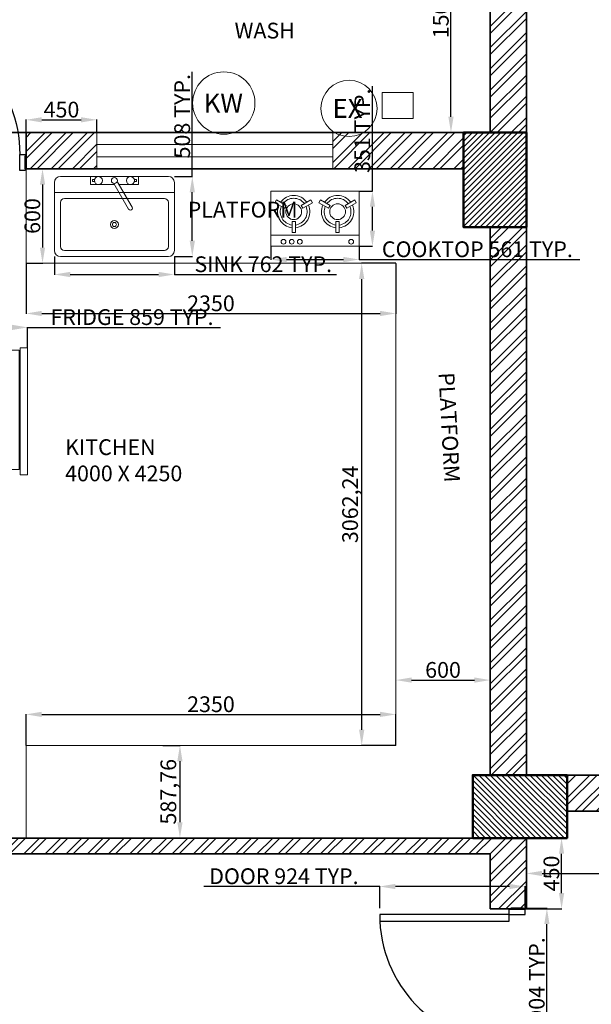
# Model space of a CAD drawing. Units: millimetres. Extents: x -3326 to 29338, y -16792 to 6002.
# Tile 10 of 21: x 8162 to 11795, y -3440 to 2813. Entities that reach past the tile are written whole.
import ezdxf

# ---------------------------------------------------------------- set-up
doc = ezdxf.new("R2010")
doc.units = ezdxf.units.MM
doc.header["$PDMODE"] = 35
doc.header["$PDSIZE"] = 5
for name, color, linetype, lineweight in [('A-ANNO-DIMS', 2, 'Continuous', 13), ('A-ANNO-SYMB', 7, 'Continuous', 18), ('A-AREA-IDEN', 7, 'Continuous', 18), ('A-COLS', 1, 'Continuous', 50), ('A-COLS-PATT', 251, 'Continuous', 13), ('A-DOOR', 3, 'Continuous', 25), ('A-EQPM', 9, 'Continuous', 18), ('A-FLOR-CASE', 30, 'Continuous', 18), ('A-FLOR-FIXT', 9, 'Continuous', 18), ('A-GLAZ', 4, 'Continuous', 18), ('A-WALL', 7, 'Continuous', 35), ('A-WALL-PATT', 252, 'Continuous', 13), ('txt', 7, 'Continuous', 18)]:
    doc.layers.add(name, color=color, linetype=linetype, lineweight=lineweight)
doc.styles.get("Standard").update_dxf_attribs({"font": 'arial.ttf'})
doc.dimstyles.new('ISO-25', dxfattribs={"dimtxt": 100, "dimasz": 100, "dimexe": 1.25, "dimexo": 0.625, "dimtad": 1, "dimtxsty": 'Standard', "dimcen": 2.5, "dimadec": 0, "dimazin": 0, "dimtfac": 1, "dimtmove": 0, "dimatfit": 3, "dimfxl": 1, "dimarcsym": 0})
pattern_1 = [(45, (-10476.65, 1e-12), (-67.35192, 67.35192), []), (45, (-10431.74, 1e-12), (-67.35192, 67.35192), [])]

# ---------------------------------------------------------------- blocks, each defined once
blk = doc.blocks.new('A$C0CE462CD')
for p, q in [((860, 100), (860, 0)), ((860, 0), (893.9, 0))]:
    blk.add_line(p, q)
for points in [[(860, 100), (860, 920), (818.4, 920), (818.4, 100)], [(0, 10), (6.1, 10), (6.1, 90), (0, 90)], [(893.9, 10), (900, 10), (900, 90), (893.9, 90)]]:
    blk.add_lwpolyline(points, close=True)
for points in [[(6.1, 0), (40, 0), (40, 100), (6.1, 100)], [(6.1, 100), (6.1, 0)], [(860, 100), (893.9, 100), (893.9, 0)]]:
    blk.add_lwpolyline(points)
blk.add_arc((859.1, 101.9), 819.1, 92.8508, 180.13091)
blk = doc.blocks.new('Sink-single - 30 in top')
blk.add_line((-15, -3.999996), (15, -3.999996))
for points in [[(-13.5, 0), (13.5, 0)], [(-15, -18.499996), (-15, -1.5)], [(15, -1.5), (15, -18.499996)], [(-13.5, -17.499996), (-13.5, -6.499996)], [(-12.5, -5.499996), (12.5, -5.499996)], [(13.5, -6.499996), (13.5, -17.499996)], [(12.5, -18.499996), (-12.5, -18.499996)], [(13.5, -19.999996), (-13.5, -19.999996)]]:
    blk.add_lwpolyline(points)
for radius in [1, 0.5]:
    blk.add_circle((0, -11.999996), radius)
for centre, radius, start, end in [((-13.5, -1.5), 1.5, 90, 180), ((13.5, -1.5), 1.5, 0, 90), ((-12.5, -6.499996), 1, 90, 180), ((12.5, -6.499996), 1, 0, 90), ((-13.5, -18.499996), 1.5, 180, 270), ((-12.5, -17.499996), 1, 180, 270), ((12.5, -17.499996), 1, 270, 0), ((13.5, -18.499996), 1.5, 270, 0)]:
    blk.add_arc(centre, radius, start, end)
blk = doc.blocks.new('Faucet - kit sink top')
for p, q in [((-5.5, -0.75), (-5.5, -1.25)), ((-4.94278, -0.75), (-5.5, -0.75)), ((-5.5, -1.25), (-4.94278, -1.25)), ((-0.14775, -1.7441), (3.56698, -8.1782)), ((4.43301, -7.6782), (0.71828, -1.2441)), ((4.94278, -0.75), (5.5, -0.75)), ((5.5, -1.25), (4.94278, -1.25)), ((5.5, -0.75), (5.5, -1.25))]:
    blk.add_line(p, q)
blk.add_lwpolyline([(-0.00587, -2), (-6, -2), (-6, 0), (6, 0), (6, -2), (1.15195, -2)])
for centre, radius in [((-4, -1), 1), ((4, -1), 1), ((0, -1), 0.75)]:
    blk.add_circle(centre, radius)
blk.add_arc((4, -7.9282), 0.5, 210, 30)
blk = doc.blocks.new('*D50')
at = {"layer": 'A-ANNO-DIMS', "color": 0, "lineweight": -2, "transparency": 16777216}
for p, q in [((11382.3, -2608.3), (11382.3, -2607.7)), ((11482.3, -2609), (17182.3, -2609)), ((17282.3, -2608.3), (17282.3, -2607.7))]:
    blk.add_line(p, q, dxfattribs=at)
at = {"layer": 'A-ANNO-DIMS', "color": 0, "transparency": 16777216}
for points in [[(11482.3, -2592.3), (11482.3, -2625.6), (11382.3, -2609)], [(17182.3, -2592.3), (17182.3, -2625.6), (17282.3, -2609)]]:
    blk.add_solid(points, dxfattribs=at)
at = {"layer": 'Defpoints', "color": 0, "transparency": 16777216}
for p in [(11382.3, -2609), (17282.3, -2609), (17282.3, -2609)]:
    blk.add_point(p, dxfattribs=at)
at = {"layer": 'A-ANNO-DIMS', "color": 0, "transparency": 16777216, "insert": (14332.3, -2557.3), "char_height": 100, "attachment_point": 5}
blk.add_mtext('5900', dxfattribs=at)
blk = doc.blocks.new('*D51')
at = {"layer": 'A-ANNO-DIMS', "color": 0, "lineweight": -2, "transparency": 16777216}
for p, q in [((11382.9, -2384), (11607, -2384)), ((11605.7, -2734), (11605.7, -2484)), ((11382.9, -2834), (11607, -2834))]:
    blk.add_line(p, q, dxfattribs=at)
at = {"layer": 'A-ANNO-DIMS', "color": 0, "transparency": 16777216}
for points in [[(11589.1, -2484), (11622.4, -2484), (11605.7, -2384)], [(11589.1, -2734), (11622.4, -2734), (11605.7, -2834)]]:
    blk.add_solid(points, dxfattribs=at)
at = {"layer": 'Defpoints', "color": 0, "transparency": 16777216}
for p in [(11382.3, -2384), (11605.7, -2384), (11382.3, -2834)]:
    blk.add_point(p, dxfattribs=at)
at = {"layer": 'A-ANNO-DIMS', "color": 0, "transparency": 16777216, "insert": (11554, -2609), "char_height": 100, "attachment_point": 5, "rotation": 90}
blk.add_mtext('450', dxfattribs=at)
blk = doc.blocks.new('*D121')
at = {"layer": 'A-ANNO-DIMS', "color": 0, "lineweight": -2, "transparency": 16777216}
for p, q in [((9071.8, -1796.2), (9181.4, -1796.2)), ((9180.2, -1896.2), (9180.2, -2284)), ((9071.8, -2384), (9181.4, -2384))]:
    blk.add_line(p, q, dxfattribs=at)
at = {"layer": 'A-ANNO-DIMS', "color": 0, "transparency": 16777216}
for points in [[(9163.5, -1896.2), (9196.8, -1896.2), (9180.2, -1796.2)], [(9163.5, -2284), (9196.8, -2284), (9180.2, -2384)]]:
    blk.add_solid(points, dxfattribs=at)
at = {"layer": 'Defpoints', "color": 0, "transparency": 16777216}
for p in [(9071.2, -1796.2), (9071.2, -2384), (9180.2, -2384)]:
    blk.add_point(p, dxfattribs=at)
at = {"layer": 'A-ANNO-DIMS', "color": 0, "transparency": 16777216, "insert": (9119.4, -2090.1), "char_height": 100, "attachment_point": 5, "rotation": 90}
blk.add_mtext('587,76', dxfattribs=at)
blk = doc.blocks.new('*D122')
at = {"layer": 'A-ANNO-DIMS', "color": 0, "lineweight": -2, "transparency": 16777216}
for p, q in [((10552.3, -1380.4), (10552.3, -1379.7)), ((10652.3, -1381), (11052.3, -1381)), ((11152.3, -1380.4), (11152.3, -1379.7))]:
    blk.add_line(p, q, dxfattribs=at)
at = {"layer": 'A-ANNO-DIMS', "color": 0, "transparency": 16777216}
for points in [[(10652.3, -1364.3), (10652.3, -1397.7), (10552.3, -1381)], [(11052.3, -1364.3), (11052.3, -1397.7), (11152.3, -1381)]]:
    blk.add_solid(points, dxfattribs=at)
at = {"layer": 'Defpoints', "color": 0, "transparency": 16777216}
for p in [(10552.3, -1381), (11152.3, -1381), (11152.3, -1381)]:
    blk.add_point(p, dxfattribs=at)
at = {"layer": 'A-ANNO-DIMS', "color": 0, "transparency": 16777216, "insert": (10852.3, -1329.3), "char_height": 100, "attachment_point": 5}
blk.add_mtext('600', dxfattribs=at)
blk = doc.blocks.new('*D123')
at = {"layer": 'A-ANNO-DIMS', "color": 0, "lineweight": -2, "transparency": 16777216}
for p, q in [((8202.9, 1866), (8308, 1866)), ((8306.8, 1766), (8306.8, 1366)), ((8202.9, 1266), (8308, 1266))]:
    blk.add_line(p, q, dxfattribs=at)
at = {"layer": 'A-ANNO-DIMS', "color": 0, "transparency": 16777216}
for points in [[(8290.1, 1766), (8323.5, 1766), (8306.8, 1866)], [(8290.1, 1366), (8323.5, 1366), (8306.8, 1266)]]:
    blk.add_solid(points, dxfattribs=at)
at = {"layer": 'Defpoints', "color": 0, "transparency": 16777216}
for p in [(8202.3, 1866), (8202.3, 1266), (8306.8, 1266)]:
    blk.add_point(p, dxfattribs=at)
at = {"layer": 'A-ANNO-DIMS', "color": 0, "transparency": 16777216, "insert": (8255.1, 1566), "char_height": 100, "attachment_point": 5, "rotation": 90}
blk.add_mtext('600', dxfattribs=at)
blk = doc.blocks.new('*D124')
at = {"layer": 'A-ANNO-DIMS', "color": 0, "lineweight": -2, "transparency": 16777216}
for p, q in [((8202.3, 1265.4), (8202.3, 945.9)), ((10552.3, 1265.4), (10552.3, 945.9)), ((8302.3, 947.1), (10452.3, 947.1))]:
    blk.add_line(p, q, dxfattribs=at)
at = {"layer": 'A-ANNO-DIMS', "color": 0, "transparency": 16777216}
for points in [[(8302.3, 963.8), (8302.3, 930.5), (8202.3, 947.1)], [(10452.3, 963.8), (10452.3, 930.5), (10552.3, 947.1)]]:
    blk.add_solid(points, dxfattribs=at)
at = {"layer": 'Defpoints', "color": 0, "transparency": 16777216}
for p in [(8202.3, 1266), (10552.3, 1266), (10552.3, 947.1)]:
    blk.add_point(p, dxfattribs=at)
at = {"layer": 'A-ANNO-DIMS', "color": 0, "transparency": 16777216, "insert": (9377.3, 998.8), "char_height": 100, "attachment_point": 5}
blk.add_mtext('2350', dxfattribs=at)
blk = doc.blocks.new('*D125')
at = {"layer": 'A-ANNO-DIMS', "color": 0, "lineweight": -2, "transparency": 16777216}
for p, q in [((8202.3, -1795.6), (8202.3, -1597.6)), ((8302.3, -1598.9), (10452.3, -1598.9)), ((10552.3, -1795.6), (10552.3, -1597.6))]:
    blk.add_line(p, q, dxfattribs=at)
at = {"layer": 'A-ANNO-DIMS', "color": 0, "transparency": 16777216}
for points in [[(8302.3, -1582.2), (8302.3, -1615.5), (8202.3, -1598.9)], [(10452.3, -1582.2), (10452.3, -1615.5), (10552.3, -1598.9)]]:
    blk.add_solid(points, dxfattribs=at)
at = {"layer": 'Defpoints', "color": 0, "transparency": 16777216}
for p in [(10552.3, -1598.9), (8202.3, -1796.2), (10552.3, -1796.2)]:
    blk.add_point(p, dxfattribs=at)
at = {"layer": 'A-ANNO-DIMS', "color": 0, "transparency": 16777216, "insert": (9377.3, -1547.1), "char_height": 100, "attachment_point": 5}
blk.add_mtext('2350', dxfattribs=at)
blk = doc.blocks.new('*D126')
at = {"layer": 'A-ANNO-DIMS', "color": 0, "lineweight": -2, "transparency": 16777216}
for p, q in [((10551.7, 1266), (10334, 1266)), ((10335.3, -1696.2), (10335.3, 1166)), ((10551.7, -1796.2), (10334, -1796.2))]:
    blk.add_line(p, q, dxfattribs=at)
at = {"layer": 'A-ANNO-DIMS', "color": 0, "transparency": 16777216}
for points in [[(10318.6, 1166), (10352, 1166), (10335.3, 1266)], [(10318.6, -1696.2), (10352, -1696.2), (10335.3, -1796.2)]]:
    blk.add_solid(points, dxfattribs=at)
at = {"layer": 'Defpoints', "color": 0, "transparency": 16777216}
for p in [(10335.3, 1266), (10552.3, 1266), (10552.3, -1796.2)]:
    blk.add_point(p, dxfattribs=at)
at = {"layer": 'A-ANNO-DIMS', "color": 0, "transparency": 16777216, "insert": (10274.6, -265.1), "char_height": 100, "attachment_point": 5, "rotation": 90}
blk.add_mtext('3062,24', dxfattribs=at)
blk = doc.blocks.new('*D127')
at = {"layer": 'A-ANNO-DIMS', "color": 0, "lineweight": -2, "transparency": 16777216}
for p, q in [((11151.7, 3596), (10901.5, 3596)), ((10902.7, 2196), (10902.7, 3496)), ((11151.7, 2096), (10901.5, 2096))]:
    blk.add_line(p, q, dxfattribs=at)
at = {"layer": 'A-ANNO-DIMS', "color": 0, "transparency": 16777216}
for points in [[(10886.1, 3496), (10919.4, 3496), (10902.7, 3596)], [(10886.1, 2196), (10919.4, 2196), (10902.7, 2096)]]:
    blk.add_solid(points, dxfattribs=at)
at = {"layer": 'Defpoints', "color": 0, "transparency": 16777216}
for p in [(10902.7, 3596), (11152.3, 3596), (11152.3, 2096)]:
    blk.add_point(p, dxfattribs=at)
at = {"layer": 'A-ANNO-DIMS', "color": 0, "transparency": 16777216, "insert": (10851.1, 2846), "char_height": 100, "attachment_point": 5, "rotation": 90}
blk.add_mtext('1500', dxfattribs=at)
blk = doc.blocks.new('*D144')
at = {"layer": 'A-ANNO-DIMS', "color": 0, "lineweight": -2, "transparency": 16777216}
for p, q in [((8202.3, 2096.7), (8202.3, 2178.4)), ((8302.3, 2177.1), (8552.3, 2177.1)), ((8652.3, 2096.7), (8652.3, 2178.4))]:
    blk.add_line(p, q, dxfattribs=at)
at = {"layer": 'A-ANNO-DIMS', "color": 0, "transparency": 16777216}
for points in [[(8302.3, 2193.8), (8302.3, 2160.5), (8202.3, 2177.1)], [(8552.3, 2193.8), (8552.3, 2160.5), (8652.3, 2177.1)]]:
    blk.add_solid(points, dxfattribs=at)
at = {"layer": 'Defpoints', "color": 0, "transparency": 16777216}
for p in [(8652.3, 2177.1), (8202.3, 2096), (8652.3, 2096)]:
    blk.add_point(p, dxfattribs=at)
at = {"layer": 'A-ANNO-DIMS', "color": 0, "transparency": 16777216, "insert": (8427.3, 2228.8), "char_height": 100, "attachment_point": 5}
blk.add_mtext('450', dxfattribs=at)
blk = doc.blocks.new('COOKTOP-TWO-BURNER')
for p, q in [((561.3, 350.8), (0, 350.8)), ((0, 0), (0, 350.8)), ((561.3, 0), (561.3, 350.8)), ((26.1, 276.2), (36.6, 294.4)), ((86.6, 241.2), (26.1, 276.2)), ((97.2, 259.4), (36.6, 294.4)), ((86.6, 241.2), (97.2, 259.4)), ((193, 259.4), (253.6, 294.3)), ((193, 259.4), (203.5, 241.1)), ((203.5, 241.1), (264.1, 276.1)), ((253.6, 294.3), (264.1, 276.1)), ((305, 276.2), (315.6, 294.4)), ((365.6, 241.2), (305, 276.2)), ((376.1, 259.4), (315.6, 294.4)), ((365.6, 241.2), (376.1, 259.4)), ((472, 259.4), (532.5, 294.3)), ((472, 259.4), (482.5, 241.1)), ((482.5, 241.1), (543, 276.1)), ((532.5, 294.3), (543, 276.1)), ((134.5, 158.1), (134.5, 88.2)), ((155.6, 158.1), (134.5, 158.1)), ((155.6, 158.1), (155.5, 88.2)), ((413.5, 158.1), (413.4, 88.2)), ((434.5, 158.1), (413.5, 158.1)), ((434.5, 158.1), (434.5, 88.2)), ((561.3, 70.2), (0, 70.2)), ((155.5, 88.2), (134.5, 88.2)), ((434.5, 88.2), (413.4, 88.2)), ((561.3, 0), (0, 0))]:
    blk.add_line(p, q)
at = {"extrusion": (0, 0, -1)}
for centre, major_axis, start_param, end_param in [((145.1, 219.6), (-0.2, 102.8), -0.942584, 0.946692), ((424, 219.6), (0, 102.8), -0.944011, 0.945266), ((145.1, 219.6), (-0.1, 102.8), 3.2451, 5.134376), ((145.1, 219.6), (-60.3, 60.3), 4.051123, 5.898002), ((145.1, 219.6), (-60.3, 60.3), 6.145519, 7.992397), ((145.1, 219.6), (-35.5, 35.5), 2.356194490192311, 8.639379797371898), ((145.1, 219.6), (0.1, 102.8), 1.148752, 3.038029), ((145.1, 219.6), (60.3, 60.3), 0.385932, 2.23281), ((424, 219.6), (0, 102.8), 3.244173, 5.13345), ((424, 219.6), (60.3, 60.3), 2.480327, 4.327205), ((424, 219.6), (-60.3, 60.3), 6.145519, 7.992397), ((424, 219.6), (-35.5, 35.5), 2.356194490192306, 8.639379797371893), ((424, 219.6), (0.1, 102.8), 1.14879, 3.038067), ((424, 219.6), (60.3, 60.3), 0.385932, 2.23281), ((79.9, 28.7), (-10.8, 10.8), 2.356194490192189, 8.639379797371776), ((132.6, 28.7), (-10.8, 10.8), 2.356194490192189, 8.639379797371776), ((184.2, 28.7), (-10.8, 10.8), 2.356194490192189, 8.639379797371776), ((510, 28.7), (-10.8, 10.8), 2.356194490192189, 8.639379797371776)]:
    blk.add_ellipse(centre, major_axis=major_axis, ratio=1, start_param=start_param, end_param=end_param, dxfattribs=at)
blk = doc.blocks.new('REFRIGERATOR-PLAN')
for points in [[(0, 791.3), (804.9, 791.3), (804.9, 34.9), (0, 34.9)], [(812.5, 807.8), (859.3, 807.8), (859.3, 0), (812.5, 0)]]:
    blk.add_lwpolyline(points, close=True)
blk = doc.blocks.new('TAG-KW')
blk.add_circle((198.2, 198.2), 198.2)
at = {"insert": (70.3, 258.2), "char_height": 120, "attachment_point": 1}
blk.add_mtext_dynamic_manual_height_columns('KW', width=376.575, gutter_width=12.5, heights=[0], dxfattribs=at)
blk = doc.blocks.new('GLAZ-1500x80')
for p, q in [((0, 80), (1500, 80)), ((0, 0), (1500, 0))]:
    blk.add_line(p, q)
blk = doc.blocks.new('*D195')
at = {"layer": 'A-ANNO-DIMS', "color": 0, "lineweight": -2, "transparency": 16777216}
for p, q in [((10450.2, -2691.8), (9331.5, -2691.8)), ((10450.2, -2829.8), (10450.2, -2690.6)), ((11273.9, -2691.8), (10550.2, -2691.8)), ((11373.9, -2829.8), (11373.9, -2690.6))]:
    blk.add_line(p, q, dxfattribs=at)
at = {"layer": 'A-ANNO-DIMS', "color": 0, "transparency": 16777216}
for points in [[(10550.2, -2675.2), (10550.2, -2708.5), (10450.2, -2691.8)], [(11273.9, -2675.2), (11273.9, -2708.5), (11373.9, -2691.8)]]:
    blk.add_solid(points, dxfattribs=at)
at = {"layer": 'Defpoints', "color": 0, "transparency": 16777216}
for p in [(10450.2, -2691.8), (10450.2, -2830.4), (11373.9, -2830.4)]:
    blk.add_point(p, dxfattribs=at)
at = {"layer": 'A-ANNO-DIMS', "color": 0, "transparency": 16777216, "insert": (9840.8, -2639.5), "char_height": 100, "attachment_point": 5}
blk.add_mtext('DOOR 924 TYP.', dxfattribs=at)
blk = doc.blocks.new('*D196')
at = {"layer": 'A-ANNO-DIMS', "color": 0, "lineweight": -2, "transparency": 16777216}
for p, q in [((11374.5, -2830.4), (11513.7, -2830.4)), ((11512.5, -3634.1), (11512.5, -2930.4)), ((11374.5, -3734.1), (11513.7, -3734.1))]:
    blk.add_line(p, q, dxfattribs=at)
at = {"layer": 'A-ANNO-DIMS', "color": 0, "transparency": 16777216}
for points in [[(11495.8, -2930.4), (11529.1, -2930.4), (11512.5, -2830.4)], [(11495.8, -3634.1), (11529.1, -3634.1), (11512.5, -3734.1)]]:
    blk.add_solid(points, dxfattribs=at)
at = {"layer": 'Defpoints', "color": 0, "transparency": 16777216}
for p in [(11373.9, -2830.4), (11512.5, -2830.4), (11373.9, -3734.1)]:
    blk.add_point(p, dxfattribs=at)
at = {"layer": 'A-ANNO-DIMS', "color": 0, "transparency": 16777216, "insert": (11460.8, -3282.2), "char_height": 100, "attachment_point": 5, "rotation": 90}
blk.add_mtext('904 TYP.', dxfattribs=at)
blk = doc.blocks.new('*D221')
at = {"layer": 'A-ANNO-DIMS', "color": 0, "lineweight": -2, "transparency": 16777216}
for p, q in [((8382.6, 1308.4), (8382.6, 1193.4)), ((9144.6, 1308.4), (9144.6, 1193.4)), ((8482.6, 1194.7), (9044.6, 1194.7)), ((9144.6, 1194.7), (10174.7, 1194.7))]:
    blk.add_line(p, q, dxfattribs=at)
at = {"layer": 'A-ANNO-DIMS', "color": 0, "transparency": 16777216}
for points in [[(8482.6, 1211.3), (8482.6, 1178), (8382.6, 1194.7)], [(9044.6, 1211.3), (9044.6, 1178), (9144.6, 1194.7)]]:
    blk.add_solid(points, dxfattribs=at)
at = {"layer": 'Defpoints', "color": 0, "transparency": 16777216}
for p in [(8382.6, 1309), (9144.6, 1309), (9144.6, 1194.7)]:
    blk.add_point(p, dxfattribs=at)
at = {"layer": 'A-ANNO-DIMS', "color": 0, "transparency": 16777216, "insert": (9709.7, 1247), "char_height": 100, "attachment_point": 5}
blk.add_mtext('SINK 762 TYP.', dxfattribs=at)
blk = doc.blocks.new('*D222')
at = {"layer": 'A-ANNO-DIMS', "color": 0, "lineweight": -2, "transparency": 16777216}
for p, q in [((9258.9, 1817), (9258.9, 2482.7)), ((9145.2, 1817), (9260.2, 1817)), ((9258.9, 1409), (9258.9, 1717)), ((9145.2, 1309), (9260.2, 1309))]:
    blk.add_line(p, q, dxfattribs=at)
at = {"layer": 'A-ANNO-DIMS', "color": 0, "transparency": 16777216}
for points in [[(9242.2, 1717), (9275.6, 1717), (9258.9, 1817)], [(9242.2, 1409), (9275.6, 1409), (9258.9, 1309)]]:
    blk.add_solid(points, dxfattribs=at)
at = {"layer": 'Defpoints', "color": 0, "transparency": 16777216}
for p in [(9144.6, 1817), (9258.9, 1817), (9144.6, 1309)]:
    blk.add_point(p, dxfattribs=at)
at = {"layer": 'A-ANNO-DIMS', "color": 0, "transparency": 16777216, "insert": (9207.2, 2199.8), "char_height": 100, "attachment_point": 5, "rotation": 90}
blk.add_mtext('508 TYP.', dxfattribs=at)
blk = doc.blocks.new('*D231')
at = {"layer": 'A-ANNO-DIMS', "color": 0, "lineweight": -2, "transparency": 16777216}
for p, q in [((9758.2, 1373.4), (9758.2, 1288.5)), ((10319.5, 1373.4), (10319.5, 1288.5)), ((9858.2, 1289.8), (10219.5, 1289.8)), ((10319.5, 1289.8), (11721.4, 1289.8))]:
    blk.add_line(p, q, dxfattribs=at)
at = {"layer": 'A-ANNO-DIMS', "color": 0, "transparency": 16777216}
for points in [[(9858.2, 1306.4), (9858.2, 1273.1), (9758.2, 1289.8)], [(10219.5, 1306.4), (10219.5, 1273.1), (10319.5, 1289.8)]]:
    blk.add_solid(points, dxfattribs=at)
at = {"layer": 'Defpoints', "color": 0, "transparency": 16777216}
for p in [(9758.2, 1374), (10319.5, 1374), (10319.5, 1289.8)]:
    blk.add_point(p, dxfattribs=at)
at = {"layer": 'A-ANNO-DIMS', "color": 0, "transparency": 16777216, "insert": (11070.5, 1342.1), "char_height": 100, "attachment_point": 5}
blk.add_mtext('COOKTOP 561 TYP.', dxfattribs=at)
blk = doc.blocks.new('*D232')
at = {"layer": 'A-ANNO-DIMS', "color": 0, "lineweight": -2, "transparency": 16777216}
for p, q in [((10403.7, 1724.8), (10403.7, 2390.4)), ((10320.1, 1724.8), (10405, 1724.8)), ((10403.7, 1474), (10403.7, 1624.8)), ((10320.1, 1374), (10405, 1374))]:
    blk.add_line(p, q, dxfattribs=at)
at = {"layer": 'A-ANNO-DIMS', "color": 0, "transparency": 16777216}
for points in [[(10387, 1624.8), (10420.4, 1624.8), (10403.7, 1724.8)], [(10387, 1474), (10420.4, 1474), (10403.7, 1374)]]:
    blk.add_solid(points, dxfattribs=at)
at = {"layer": 'Defpoints', "color": 0, "transparency": 16777216}
for p in [(10319.5, 1724.8), (10403.7, 1724.8), (10319.5, 1374)]:
    blk.add_point(p, dxfattribs=at)
at = {"layer": 'A-ANNO-DIMS', "color": 0, "transparency": 16777216, "insert": (10352, 2107.6), "char_height": 100, "attachment_point": 5, "rotation": 90}
blk.add_mtext('351 TYP.', dxfattribs=at)
blk = doc.blocks.new('*D233')
at = {"layer": 'A-ANNO-DIMS', "color": 0, "lineweight": -2, "transparency": 16777216}
for p, q in [((7352.6, 730.5), (7352.6, 860.1)), ((7452.6, 858.8), (8111.9, 858.8)), ((8211.9, 730.5), (8211.9, 860.1)), ((8211.9, 858.8), (9438.5, 858.8))]:
    blk.add_line(p, q, dxfattribs=at)
at = {"layer": 'A-ANNO-DIMS', "color": 0, "transparency": 16777216}
for points in [[(7452.6, 875.5), (7452.6, 842.1), (7352.6, 858.8)], [(8111.9, 875.5), (8111.9, 842.1), (8211.9, 858.8)]]:
    blk.add_solid(points, dxfattribs=at)
at = {"layer": 'Defpoints', "color": 0, "transparency": 16777216}
for p in [(8211.9, 858.8), (7352.6, 729.9), (8211.9, 729.9)]:
    blk.add_point(p, dxfattribs=at)
at = {"layer": 'A-ANNO-DIMS', "color": 0, "transparency": 16777216, "insert": (8875.2, 911.1), "char_height": 100, "attachment_point": 5}
blk.add_mtext('FRIDGE 859 TYP.', dxfattribs=at)

msp = doc.modelspace()

# ---------------------------------------------------------------- hatches: boundary and pattern name
at = {"layer": 'A-COLS-PATT'}
h = msp.add_hatch(dxfattribs=at)
h.set_pattern_fill('ANSI31', color=256, scale=8)
h.set_pattern_definition([(45, (-30739, 8703.052), (-17.960512, 17.960512), [])])
h.paths.add_polyline_path([(10982.301, 1496.048), (11382.301, 1496.048), (11382.301, 2096.048), (10982.301, 2096.048)])
h = msp.add_hatch(dxfattribs=at)
h.set_pattern_fill('ANSI31', color=256, scale=8, angle=-90)
h.set_pattern_definition([(315, (18247.866, 39737.347), (17.960512, 17.960512), [])])
h.paths.add_polyline_path([(11040.861, -1983.952), (11040.861, -2383.952), (11640.861, -2383.952), (11640.861, -1983.952)])
at = {"layer": 'A-WALL-PATT'}
h = msp.add_hatch(dxfattribs=at)
h.set_pattern_fill('ANSI32', color=256, scale=10)
h.set_pattern_definition(pattern_1)
h.paths.add_polyline_path([(12212.301, -1983.952), (11640.861, -1983.952), (11640.861, -2213.952), (12212.301, -2213.952)])
h.paths.add_polyline_path([(14712.301, -1983.952), (14012.301, -1983.952), (14012.301, -2213.952), (14712.301, -2213.952)])
h.paths.add_polyline_path([(17012.301, -1983.952), (16512.301, -1983.952), (16512.301, -2213.952), (17012.301, -2213.952)])
h.paths.add_polyline_path([(11382.301, -2383.952), (11040.861, -2383.952), (7302.301, -2383.952), (7302.301, -1935.766), (7217.026, -1935.766), (7202.301, -1933.952), (7202.301, -2483.952), (7302.301, -2483.952), (11152.301, -2483.952), (11152.301, -2833.952), (11283.549, -2833.952), (11283.549, -2830.395), (11363.875, -2830.395), (11382.301, -2833.952)])
h.paths.add_polyline_path([(11382.301, -3733.952), (11363.875, -3733.952), (11363.875, -3734.058), (11283.549, -3734.058), (11152.301, -3733.952), (11152.301, -6450.401), (11382.301, -6450.401)])
h.paths.add_polyline_path([(13462.301, -6450.401), (12606.738, -6450.401), (11382.301, -6450.401), (11382.301, -6680.401), (12606.738, -6680.401), (13462.301, -6680.401)])
h.paths.add_polyline_path([(11382.301, -7050.401), (11152.301, -7050.401), (11152.301, -8810.401), (11382.301, -8810.401)])
h.paths.add_polyline_path([(13462.301, -8980.401), (11751.174, -8980.401), (11751.174, -9210.401), (13462.301, -9210.401)])
h.paths.add_polyline_path([(13962.301, -6850.401), (13732.301, -6850.401), (13732.301, -7350.401), (13962.301, -7350.401)])
h.paths.add_polyline_path([(13962.301, -8309.482), (13732.301, -8309.482), (13732.301, -8809.482), (13962.301, -8809.482)])
h.paths.add_polyline_path([(15712.301, -12533.952), (12902.301, -12533.952), (12902.301, -12763.952), (15712.301, -12763.952)])
h.paths.add_polyline_path([(11508.301, -9211.585), (11382.301, -9211.585), (11152.301, -9211.585), (11152.301, -11033.952), (10952.301, -11033.952), (10952.301, -11263.952), (11152.301, -11263.952), (11152.301, -12361.585), (11508.301, -12361.585)])
h.paths.add_polyline_path([(12002.301, -12533.952), (11902.301, -12533.952), (11902.301, -12761.585), (11152.301, -12761.585), (11152.301, -12763.952), (11902.301, -12763.952), (12002.301, -12763.952)])
h.paths.add_polyline_path([(17112.301, -12533.952), (16912.301, -12533.952), (16912.301, -12763.952), (17112.301, -12763.952)])
h.paths.add_polyline_path([(11382.301, 3596.048), (11152.301, 3596.048), (11152.301, 2096.048), (11382.301, 2096.048)])
h.paths.add_polyline_path([(11382.301, 1496.048), (11152.301, 1496.048), (11152.301, -1983.952), (11382.301, -1983.952)])
h = msp.add_hatch(dxfattribs=at)
h.set_pattern_fill('ANSI32', color=256, scale=10)
h.set_pattern_definition(pattern_1)
h.paths.add_polyline_path([(8652.301, 2096.048), (8202.301, 2096.048), (8202.301, 1866.048), (8652.301, 1866.048)])
h.paths.add_polyline_path([(10982.301, 2096.048), (10152.301, 2096.048), (10152.301, 1866.048), (10982.301, 1866.048)])

# ---------------------------------------------------------------- linework, layer by layer
at = {"layer": 'A-ANNO-SYMB'}
msp.add_circle((10254.723, 2249.364), 178.636, dxfattribs=at)
at = {"layer": 'A-COLS'}
for points in [[(10982.301, 2096.048), (11382.301, 2096.048), (11382.301, 1496.048), (10982.301, 1496.048)], [(11640.861, -1983.952), (11640.861, -2383.952), (11040.861, -2383.952), (11040.861, -1983.952)]]:
    msp.add_lwpolyline(points, close=True, dxfattribs=at)
at = {"layer": 'A-EQPM'}
msp.add_lwpolyline([(10465.362, 2349.703), (10661.811, 2349.703), (10661.811, 2184.867), (10465.362, 2184.867)], close=True, dxfattribs=at)
at = {"layer": 'A-FLOR-CASE'}
for p, q in [((8202.301, 1866.048), (8202.301, 1266.048)), ((8202.301, 1266.048), (10552.301, 1266.048)), ((10552.301, 1266.048), (10552.301, -1796.189)), ((10552.301, -1796.189), (8202.301, -1796.189)), ((8202.301, -1796.189), (8202.301, -2383.952))]:
    msp.add_line(p, q, dxfattribs=at)
at = {"layer": 'A-GLAZ'}
for p, q in [((8652.301, 2096.048), (8652.301, 1866.048)), ((10152.301, 2096.048), (10152.301, 1866.048))]:
    msp.add_line(p, q, dxfattribs=at)
at = {"layer": 'A-WALL'}
for p, q in [((11152.301, 3596.048), (11152.301, 2096.048)), ((11382.301, 3596.048), (11382.301, -1983.952)), ((10982.301, 2096.048), (7302.301, 2096.048)), ((8202.301, 2096.048), (8202.301, 1866.048)), ((10982.301, 1866.048), (8202.301, 1866.048)), ((11152.301, 1496.048), (11152.301, -1983.952)), ((17012.301, -1983.952), (11640.861, -1983.952)), ((17012.301, -2213.952), (11640.861, -2213.952)), ((11152.301, -2383.952), (7302.301, -2383.952)), ((11382.301, -2383.952), (11382.301, -2833.952)), ((11152.301, -2483.952), (7302.301, -2483.952)), ((11152.301, -2483.952), (11152.301, -2833.952)), ((11382.301, -2833.952), (11152.301, -2833.952))]:
    msp.add_line(p, q, dxfattribs=at)

# ---------------------------------------------------------------- block references
at = {"layer": 'A-ANNO-SYMB'}
msp.add_blockref('TAG-KW', (9260.815, 2085.197), dxfattribs=at)
at = {"layer": 'A-DOOR', "xscale": -1}
msp.add_blockref('A$C0CE462CD', (8202.301, 1856.048), dxfattribs=at)
at = {"layer": 'A-DOOR', "xscale": 1.004070386304363, "yscale": 1.004070386304363, "zscale": 1.004070386304363, "rotation": 90.00000000000003}
msp.add_blockref('A$C0CE462CD', (11373.915, -3734.058), dxfattribs=at)
at = {"layer": 'A-EQPM'}
for name, p in [('COOKTOP-TWO-BURNER', (9758.197, 1373.976)), ('REFRIGERATOR-PLAN', (7352.616, -77.917))]:
    msp.add_blockref(name, p, dxfattribs=at)
at = {"layer": 'A-FLOR-FIXT', "xscale": 25.4, "yscale": 25.4, "zscale": 25.4}
for name in ['Sink-single - 30 in top', 'Faucet - kit sink top']:
    msp.add_blockref(name, (8763.609, 1816.976), dxfattribs=at)
at = {"layer": 'A-GLAZ'}
msp.add_blockref('GLAZ-1500x80', (8652.301, 1941.048), dxfattribs=at)

# ---------------------------------------------------------------- texts
at = {"layer": 'A-ANNO-SYMB', "insert": (10150.071, 2309.364), "char_height": 120, "attachment_point": 1}
msp.add_mtext_dynamic_manual_height_columns('EX', width=92.17276, gutter_width=12.5, heights=[0], dxfattribs=at)
at = {"layer": 'A-AREA-IDEN', "char_height": 100, "attachment_point": 1}
for s, width, insert in [('WASH', 1168.90663, (9527.411, 2793.605)), ('KITCHEN\\P4000 X 4250', 1169.99756, (8450.302, 148.256))]:
    msp.add_mtext_dynamic_manual_height_columns(s, width=width, gutter_width=12.5, heights=[0], dxfattribs=dict(at, insert=insert))
at = {"layer": 'txt', "insert": (9229.368, 1656.445), "char_height": 100, "attachment_point": 1}
msp.add_mtext_dynamic_manual_height_columns('PLATFORM', width=464.35481, gutter_width=12.5, heights=[0], dxfattribs=at)
at = {"layer": 'txt', "insert": (10923.526, 575.527), "char_height": 100, "attachment_point": 1, "rotation": 273.041507}
msp.add_mtext_dynamic_manual_height_columns('PLATFORM', width=464.35481, gutter_width=12.5, heights=[0], dxfattribs=at)

# ---------------------------------------------------------------- dimensions: what is measured, and where the dimension line sits
at = {"layer": 'A-ANNO-DIMS'}
for base, p1, p2, picture, middle in [((10902.735, 3596.048), (11152.301, 2096.048), (11152.301, 3596.048), '*D127', (10851.053, 2846.048)), ((8306.796, 1266.048), (8202.301, 1866.048), (8202.301, 1266.048), '*D123', (8255.113, 1566.048)), ((10335.298, 1266.048), (10552.301, -1796.189), (10552.301, 1266.048), '*D126', (10274.578, -265.071)), ((9180.161, -2383.952), (9071.202, -1796.189), (9071.202, -2383.952), '*D121', (9119.44, -2090.071)), ((11605.728, -2383.952), (11382.301, -2833.952), (11382.301, -2383.952), '*D51', (11554.046, -2608.952))]:
    dim = msp.add_linear_dim(base=base, p1=p1, p2=p2, angle=90, dimstyle='ISO-25', override={"dimclrd": 0, "dimclre": 0, "dimclrt": 0}, dxfattribs=at)
    dim.commit()
    dim.dimension.update_dxf_attribs({"geometry": picture, "text_midpoint": middle})
for base, p1, p2, angle, text, picture, middle in [((9258.909, 1816.976), (9144.609, 1308.976), (9144.609, 1816.976), 90, '<> TYP.', '*D222', (9207.227, 2199.832)), ((10403.701, 1724.794), (10319.505, 1373.976), (10319.505, 1724.794), 90, '<> TYP.', '*D232', (10351.985, 2107.615)), ((10450.171, -2691.833), (11373.915, -2830.395), (10450.171, -2830.395), 180, 'DOOR <> TYP.', '*D195', (9840.848, -2639.469)), ((11512.477, -2830.395), (11373.915, -3734.058), (11373.915, -2830.395), 90, '<> TYP.', '*D196', (11460.795, -3282.227))]:
    dim = msp.add_linear_dim(base=base, p1=p1, p2=p2, angle=angle, text=text, dimstyle='ISO-25', override={"dimdec": 0, "dimlfac": 1, "dimrnd": 0, "dimzin": 0, "dimdsep": 46, "dimlunit": 2}, dxfattribs=at)
    dim.commit()
    dim.dimension.update_dxf_attribs({"geometry": picture, "text_midpoint": middle})
for base, p1, p2, picture, middle in [((8652.301, 2177.146), (8202.301, 2096.048), (8652.301, 2096.048), '*D144', (8427.301, 2228.828)), ((10552.301, 947.119), (8202.301, 1266.048), (10552.301, 1266.048), '*D124', (9377.301, 998.836)), ((11152.301, -1380.989), (10552.301, -1380.989), (11152.301, -1380.989), '*D122', (10852.301, -1329.306)), ((10552.301, -1598.853), (8202.301, -1796.189), (10552.301, -1796.189), '*D125', (9377.301, -1547.136)), ((17282.301, -2608.952), (11382.301, -2608.952), (17282.301, -2608.952), '*D50', (14332.301, -2557.27))]:
    dim = msp.add_linear_dim(base=base, p1=p1, p2=p2, dimstyle='ISO-25', override={"dimclrd": 0, "dimclre": 0, "dimclrt": 0}, dxfattribs=at)
    dim.commit()
    dim.dimension.update_dxf_attribs({"geometry": picture, "text_midpoint": middle})
for base, p1, p2, text, picture, middle in [((10319.505, 1289.78), (9758.197, 1373.976), (10319.505, 1373.976), 'COOKTOP <> TYP.', '*D231', (11070.471, 1342.144)), ((9144.609, 1194.676), (8382.609, 1308.976), (9144.609, 1308.976), 'SINK <> TYP.', '*D221', (9709.661, 1247.007)), ((8211.889, 858.805), (7352.616, 729.914), (8211.889, 729.914), 'FRIDGE <> TYP.', '*D233', (8875.201, 911.135))]:
    dim = msp.add_linear_dim(base=base, p1=p1, p2=p2, text=text, dimstyle='ISO-25', override={"dimdec": 0, "dimlfac": 1, "dimrnd": 0, "dimzin": 0, "dimdsep": 46, "dimlunit": 2}, dxfattribs=at)
    dim.commit()
    dim.dimension.update_dxf_attribs({"geometry": picture, "text_midpoint": middle})

doc.saveas('drawing.dxf')
